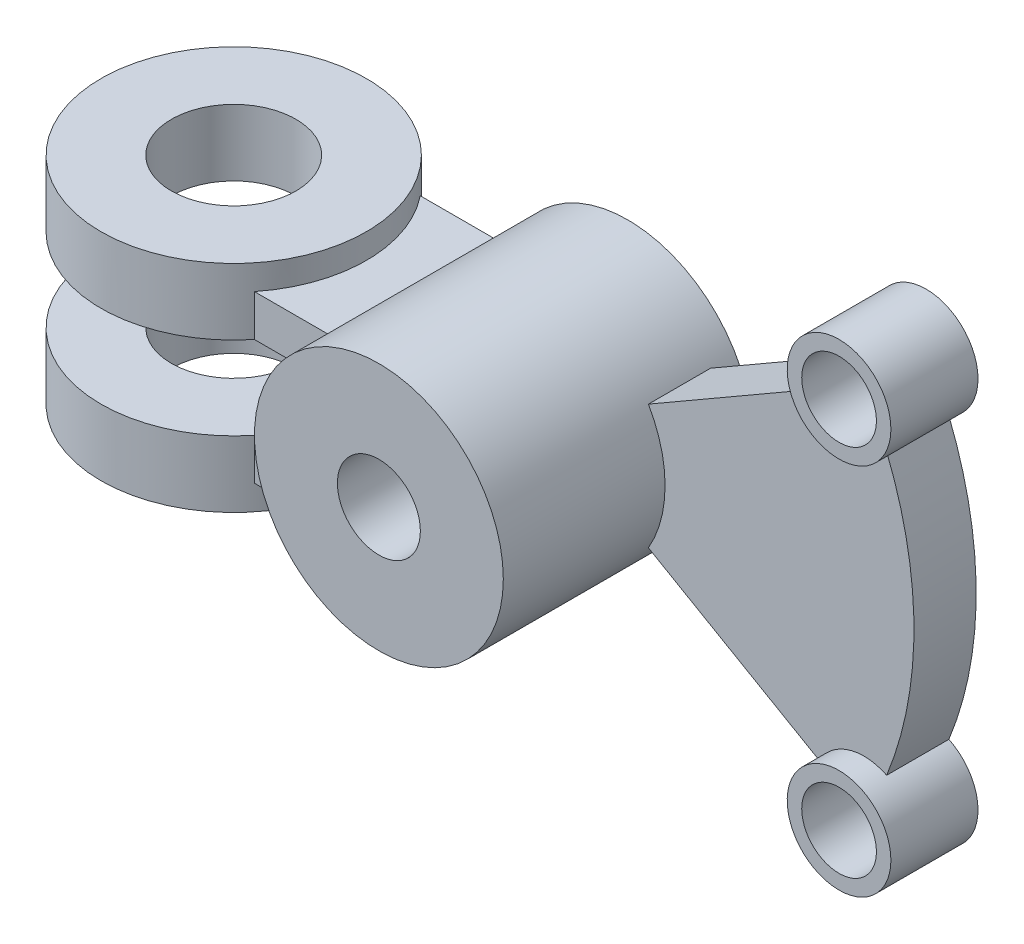
ISO-10303-21;
HEADER;
FILE_DESCRIPTION(('STEP AP214'),'2;1');
FILE_NAME('part.step','',(''),(''),'','','');
FILE_SCHEMA(('AUTOMOTIVE_DESIGN { 1 0 10303 214 1 1 1 1 }'));
ENDSEC;
DATA;
#1=APPLICATION_CONTEXT('core data for automotive mechanical design processes');
#2=APPLICATION_PROTOCOL_DEFINITION('international standard','automotive_design',2000,#1);
#3=PRODUCT_CONTEXT('',#1,'mechanical');
#4=PRODUCT('Part','Part','',(#3));
#5=PRODUCT_RELATED_PRODUCT_CATEGORY('part','',(#4));
#6=PRODUCT_DEFINITION_FORMATION('','',#4);
#7=PRODUCT_DEFINITION_CONTEXT('part definition',#1,'design');
#8=PRODUCT_DEFINITION('design','',#6,#7);
#9=PRODUCT_DEFINITION_SHAPE('','',#8);
#10=(LENGTH_UNIT() NAMED_UNIT(*) SI_UNIT(.MILLI.,.METRE.));
#11=(NAMED_UNIT(*) PLANE_ANGLE_UNIT() SI_UNIT($,.RADIAN.));
#12=(NAMED_UNIT(*) SI_UNIT($,.STERADIAN.) SOLID_ANGLE_UNIT());
#13=UNCERTAINTY_MEASURE_WITH_UNIT(LENGTH_MEASURE(1.E-05),#10,'distance_accuracy_value','');
#14=(GEOMETRIC_REPRESENTATION_CONTEXT(3) GLOBAL_UNCERTAINTY_ASSIGNED_CONTEXT((#13)) GLOBAL_UNIT_ASSIGNED_CONTEXT((#10,
#11,#12)) REPRESENTATION_CONTEXT('',''));
#15=CARTESIAN_POINT('',(0.,0.,0.));
#16=DIRECTION('',(0.,0.,1.));
#17=DIRECTION('',(1.,0.,0.));
#18=AXIS2_PLACEMENT_3D('',#15,#16,#17);
#19=CARTESIAN_POINT('',(0.,0.,21.));
#20=DIRECTION('',(0.,0.,-1.));
#21=DIRECTION('',(-1.,0.,0.));
#22=AXIS2_PLACEMENT_3D('',#19,#20,#21);
#23=CYLINDRICAL_SURFACE('',#22,90.);
#24=DIRECTION('',(0.,0.,-1.));
#25=VECTOR('',#24,1.);
#26=CARTESIAN_POINT('',(83.4254395553197,-33.7667889353089,16.5));
#27=LINE('',#26,#25);
#28=CARTESIAN_POINT('',(83.4254395553198,-33.7667889353088,6.));
#29=VERTEX_POINT('',#28);
#30=CARTESIAN_POINT('',(83.4254395553198,-33.7667889353088,21.));
#31=VERTEX_POINT('',#30);
#32=EDGE_CURVE('E374',#29,#31,#27,.F.);
#33=ORIENTED_EDGE('',*,*,#32,.F.);
#34=CARTESIAN_POINT('',(0.,0.,6.));
#35=DIRECTION('',(0.,0.,1.));
#36=DIRECTION('',(1.,0.,0.));
#37=AXIS2_PLACEMENT_3D('',#34,#35,#36);
#38=CIRCLE('',#37,90.);
#39=CARTESIAN_POINT('',(83.4254395553198,33.7667889353088,6.));
#40=VERTEX_POINT('',#39);
#41=EDGE_CURVE('E213',#29,#40,#38,.T.);
#42=ORIENTED_EDGE('',*,*,#41,.T.);
#43=DIRECTION('',(0.,0.,-1.));
#44=VECTOR('',#43,1.);
#45=CARTESIAN_POINT('',(83.4254395553198,33.7667889353089,16.5));
#46=LINE('',#45,#44);
#47=CARTESIAN_POINT('',(83.4254395553198,33.7667889353088,21.));
#48=VERTEX_POINT('',#47);
#49=EDGE_CURVE('E200',#48,#40,#46,.T.);
#50=ORIENTED_EDGE('',*,*,#49,.F.);
#51=CARTESIAN_POINT('',(0.,0.,21.));
#52=DIRECTION('',(0.,0.,1.));
#53=DIRECTION('',(1.,0.,0.));
#54=AXIS2_PLACEMENT_3D('',#51,#52,#53);
#55=CIRCLE('',#54,90.);
#56=EDGE_CURVE('E210',#31,#48,#55,.T.);
#57=ORIENTED_EDGE('',*,*,#56,.F.);
#58=EDGE_LOOP('',(#33,#42,#50,#57));
#59=FACE_BOUND('',#58,.T.);
#60=ADVANCED_FACE('F39',(#59),#23,.T.);
#61=CARTESIAN_POINT('',(0.,0.,21.));
#62=DIRECTION('',(0.500000000000001,0.866025403784438,0.));
#63=DIRECTION('',(-0.866025403784438,0.500000000000001,0.));
#64=AXIS2_PLACEMENT_3D('',#61,#62,#63);
#65=PLANE('',#64);
#66=DIRECTION('',(0.,0.,-1.));
#67=VECTOR('',#66,1.);
#68=CARTESIAN_POINT('',(67.116968793294,-38.7500000000001,27.));
#69=LINE('',#68,#67);
#70=CARTESIAN_POINT('',(67.116968793294,-38.7500000000001,21.));
#71=VERTEX_POINT('',#70);
#72=CARTESIAN_POINT('',(67.116968793294,-38.7500000000001,6.));
#73=VERTEX_POINT('',#72);
#74=EDGE_CURVE('E54',#71,#73,#69,.T.);
#75=ORIENTED_EDGE('',*,*,#74,.F.);
#76=DIRECTION('',(0.866025403784438,-0.500000000000001,0.));
#77=VECTOR('',#76,1.);
#78=CARTESIAN_POINT('',(0.,0.,21.));
#79=LINE('',#78,#77);
#80=CARTESIAN_POINT('',(25.9807621135331,-15.,21.));
#81=VERTEX_POINT('',#80);
#82=EDGE_CURVE('E201',#81,#71,#79,.T.);
#83=ORIENTED_EDGE('',*,*,#82,.F.);
#84=DIRECTION('',(0.,0.,-1.));
#85=VECTOR('',#84,1.);
#86=CARTESIAN_POINT('',(25.9807621135331,-15.,60.));
#87=LINE('',#86,#85);
#88=CARTESIAN_POINT('',(25.9807621135331,-15.,6.));
#89=VERTEX_POINT('',#88);
#90=EDGE_CURVE('E226',#81,#89,#87,.T.);
#91=ORIENTED_EDGE('',*,*,#90,.T.);
#92=DIRECTION('',(0.866025403784438,-0.500000000000001,0.));
#93=VECTOR('',#92,1.);
#94=CARTESIAN_POINT('',(0.,0.,6.));
#95=LINE('',#94,#93);
#96=EDGE_CURVE('E204',#89,#73,#95,.T.);
#97=ORIENTED_EDGE('',*,*,#96,.T.);
#98=EDGE_LOOP('',(#75,#83,#91,#97));
#99=FACE_BOUND('',#98,.T.);
#100=ADVANCED_FACE('F321',(#99),#65,.F.);
#101=CARTESIAN_POINT('',(-22.0435348575211,20.,50.));
#102=DIRECTION('',(0.,0.,-1.));
#103=DIRECTION('',(-1.,0.,0.));
#104=AXIS2_PLACEMENT_3D('',#101,#102,#103);
#105=PLANE('',#104);
#106=DIRECTION('',(0.,-1.,0.));
#107=VECTOR('',#106,1.);
#108=CARTESIAN_POINT('',(-40.0200080064064,26.,50.));
#109=LINE('',#108,#107);
#110=CARTESIAN_POINT('',(-40.0200080064064,10.,50.));
#111=VERTEX_POINT('',#110);
#112=CARTESIAN_POINT('',(-40.0200080064064,20.,50.));
#113=VERTEX_POINT('',#112);
#114=EDGE_CURVE('E167',#111,#113,#109,.F.);
#115=ORIENTED_EDGE('',*,*,#114,.F.);
#116=DIRECTION('',(1.,0.,0.));
#117=VECTOR('',#116,1.);
#118=CARTESIAN_POINT('',(-22.0435348575211,10.,50.));
#119=LINE('',#118,#117);
#120=CARTESIAN_POINT('',(-28.2842712474619,10.,50.));
#121=VERTEX_POINT('',#120);
#122=EDGE_CURVE('E181',#111,#121,#119,.T.);
#123=ORIENTED_EDGE('',*,*,#122,.T.);
#124=CARTESIAN_POINT('',(0.,0.,50.));
#125=DIRECTION('',(0.,0.,-1.));
#126=DIRECTION('',(-1.,0.,0.));
#127=AXIS2_PLACEMENT_3D('',#124,#125,#126);
#128=CIRCLE('',#127,30.);
#129=CARTESIAN_POINT('',(-22.3606797749979,20.,50.));
#130=VERTEX_POINT('',#129);
#131=EDGE_CURVE('E239',#121,#130,#128,.T.);
#132=ORIENTED_EDGE('',*,*,#131,.T.);
#133=DIRECTION('',(1.,0.,0.));
#134=VECTOR('',#133,1.);
#135=CARTESIAN_POINT('',(-80.,20.,50.));
#136=LINE('',#135,#134);
#137=EDGE_CURVE('E172',#113,#130,#136,.T.);
#138=ORIENTED_EDGE('',*,*,#137,.F.);
#139=EDGE_LOOP('',(#115,#123,#132,#138));
#140=FACE_BOUND('',#139,.T.);
#141=ADVANCED_FACE('F279',(#140),#105,.F.);
#142=CARTESIAN_POINT('',(-80.,20.,10.));
#143=DIRECTION('',(0.,0.,1.));
#144=DIRECTION('',(1.,0.,0.));
#145=AXIS2_PLACEMENT_3D('',#142,#143,#144);
#146=PLANE('',#145);
#147=DIRECTION('',(0.,-1.,0.));
#148=VECTOR('',#147,1.);
#149=CARTESIAN_POINT('',(-40.0200080064064,26.,9.99999999999999));
#150=LINE('',#149,#148);
#151=CARTESIAN_POINT('',(-40.0200080064064,20.,9.99999999999999));
#152=VERTEX_POINT('',#151);
#153=CARTESIAN_POINT('',(-40.0200080064064,10.,9.99999999999999));
#154=VERTEX_POINT('',#153);
#155=EDGE_CURVE('E48',#152,#154,#150,.T.);
#156=ORIENTED_EDGE('',*,*,#155,.F.);
#157=DIRECTION('',(-1.,0.,0.));
#158=VECTOR('',#157,1.);
#159=CARTESIAN_POINT('',(-29.7437728993575,20.,10.));
#160=LINE('',#159,#158);
#161=CARTESIAN_POINT('',(-22.3606797749979,20.,9.99999999999999));
#162=VERTEX_POINT('',#161);
#163=EDGE_CURVE('E176',#162,#152,#160,.T.);
#164=ORIENTED_EDGE('',*,*,#163,.F.);
#165=CARTESIAN_POINT('',(0.,0.,9.99999999999999));
#166=DIRECTION('',(0.,0.,1.));
#167=DIRECTION('',(1.,0.,0.));
#168=AXIS2_PLACEMENT_3D('',#165,#166,#167);
#169=CIRCLE('',#168,30.);
#170=CARTESIAN_POINT('',(-28.2842712474619,10.,9.99999999999999));
#171=VERTEX_POINT('',#170);
#172=EDGE_CURVE('E240',#162,#171,#169,.T.);
#173=ORIENTED_EDGE('',*,*,#172,.T.);
#174=DIRECTION('',(-1.,0.,0.));
#175=VECTOR('',#174,1.);
#176=CARTESIAN_POINT('',(-80.,10.,10.));
#177=LINE('',#176,#175);
#178=EDGE_CURVE('E180',#171,#154,#177,.T.);
#179=ORIENTED_EDGE('',*,*,#178,.T.);
#180=EDGE_LOOP('',(#156,#164,#173,#179));
#181=FACE_BOUND('',#180,.T.);
#182=ADVANCED_FACE('F272',(#181),#146,.F.);
#183=CARTESIAN_POINT('',(0.,0.,21.));
#184=DIRECTION('',(0.500000000000001,-0.866025403784438,0.));
#185=DIRECTION('',(0.866025403784438,0.500000000000001,0.));
#186=AXIS2_PLACEMENT_3D('',#183,#184,#185);
#187=PLANE('',#186);
#188=DIRECTION('',(0.,0.,-1.));
#189=VECTOR('',#188,1.);
#190=CARTESIAN_POINT('',(67.116968793294,38.7500000000001,27.));
#191=LINE('',#190,#189);
#192=CARTESIAN_POINT('',(67.116968793294,38.7500000000001,6.));
#193=VERTEX_POINT('',#192);
#194=CARTESIAN_POINT('',(67.116968793294,38.7500000000001,21.));
#195=VERTEX_POINT('',#194);
#196=EDGE_CURVE('E202',#193,#195,#191,.F.);
#197=ORIENTED_EDGE('',*,*,#196,.F.);
#198=DIRECTION('',(-0.866025403784438,-0.500000000000001,0.));
#199=VECTOR('',#198,1.);
#200=CARTESIAN_POINT('',(0.,0.,6.));
#201=LINE('',#200,#199);
#202=CARTESIAN_POINT('',(25.9807621135331,15.,6.));
#203=VERTEX_POINT('',#202);
#204=EDGE_CURVE('E206',#193,#203,#201,.T.);
#205=ORIENTED_EDGE('',*,*,#204,.T.);
#206=DIRECTION('',(0.,0.,-1.));
#207=VECTOR('',#206,1.);
#208=CARTESIAN_POINT('',(25.9807621135331,15.,60.));
#209=LINE('',#208,#207);
#210=CARTESIAN_POINT('',(25.9807621135331,15.,21.));
#211=VERTEX_POINT('',#210);
#212=EDGE_CURVE('E221',#203,#211,#209,.F.);
#213=ORIENTED_EDGE('',*,*,#212,.T.);
#214=DIRECTION('',(-0.866025403784438,-0.500000000000001,0.));
#215=VECTOR('',#214,1.);
#216=CARTESIAN_POINT('',(0.,0.,21.));
#217=LINE('',#216,#215);
#218=EDGE_CURVE('E208',#195,#211,#217,.T.);
#219=ORIENTED_EDGE('',*,*,#218,.F.);
#220=EDGE_LOOP('',(#197,#205,#213,#219));
#221=FACE_BOUND('',#220,.T.);
#222=ADVANCED_FACE('F327',(#221),#187,.F.);
#223=CARTESIAN_POINT('',(0.,0.,60.));
#224=DIRECTION('',(0.,0.,-1.));
#225=DIRECTION('',(-1.,0.,0.));
#226=AXIS2_PLACEMENT_3D('',#223,#224,#225);
#227=CYLINDRICAL_SURFACE('',#226,30.);
#228=CARTESIAN_POINT('',(0.,0.,50.));
#229=DIRECTION('',(0.,0.,1.));
#230=DIRECTION('',(1.,0.,0.));
#231=AXIS2_PLACEMENT_3D('',#228,#229,#230);
#232=CIRCLE('',#231,30.);
#233=CARTESIAN_POINT('',(-28.2842712474619,-10.,50.));
#234=VERTEX_POINT('',#233);
#235=CARTESIAN_POINT('',(-22.3606797749979,-20.,50.));
#236=VERTEX_POINT('',#235);
#237=EDGE_CURVE('E165',#234,#236,#232,.T.);
#238=ORIENTED_EDGE('',*,*,#237,.T.);
#239=DIRECTION('',(0.,0.,-1.));
#240=VECTOR('',#239,1.);
#241=CARTESIAN_POINT('',(-22.3606797749979,-20.,60.));
#242=LINE('',#241,#240);
#243=CARTESIAN_POINT('',(-22.3606797749979,-20.,9.99999999999999));
#244=VERTEX_POINT('',#243);
#245=EDGE_CURVE('E252',#236,#244,#242,.T.);
#246=ORIENTED_EDGE('',*,*,#245,.T.);
#247=CARTESIAN_POINT('',(0.,0.,9.99999999999999));
#248=DIRECTION('',(0.,0.,-1.));
#249=DIRECTION('',(-1.,0.,0.));
#250=AXIS2_PLACEMENT_3D('',#247,#248,#249);
#251=CIRCLE('',#250,30.);
#252=CARTESIAN_POINT('',(-28.2842712474619,-10.,10.));
#253=VERTEX_POINT('',#252);
#254=EDGE_CURVE('E248',#244,#253,#251,.T.);
#255=ORIENTED_EDGE('',*,*,#254,.T.);
#256=DIRECTION('',(0.,0.,-1.));
#257=VECTOR('',#256,1.);
#258=CARTESIAN_POINT('',(-28.2842712474619,-10.,60.));
#259=LINE('',#258,#257);
#260=EDGE_CURVE('E246',#234,#253,#259,.T.);
#261=ORIENTED_EDGE('',*,*,#260,.F.);
#262=EDGE_LOOP('',(#238,#246,#255,#261));
#263=FACE_BOUND('',#262,.T.);
#264=ORIENTED_EDGE('',*,*,#172,.F.);
#265=DIRECTION('',(0.,0.,-1.));
#266=VECTOR('',#265,1.);
#267=CARTESIAN_POINT('',(-22.3606797749979,20.,60.));
#268=LINE('',#267,#266);
#269=EDGE_CURVE('E243',#162,#130,#268,.F.);
#270=ORIENTED_EDGE('',*,*,#269,.T.);
#271=ORIENTED_EDGE('',*,*,#131,.F.);
#272=DIRECTION('',(0.,0.,-1.));
#273=VECTOR('',#272,1.);
#274=CARTESIAN_POINT('',(-28.2842712474619,10.,60.));
#275=LINE('',#274,#273);
#276=EDGE_CURVE('E234',#171,#121,#275,.F.);
#277=ORIENTED_EDGE('',*,*,#276,.F.);
#278=EDGE_LOOP('',(#264,#270,#271,#277));
#279=FACE_BOUND('',#278,.T.);
#280=ORIENTED_EDGE('',*,*,#90,.F.);
#281=CARTESIAN_POINT('',(0.,0.,21.));
#282=DIRECTION('',(0.,0.,1.));
#283=DIRECTION('',(1.,0.,0.));
#284=AXIS2_PLACEMENT_3D('',#281,#282,#283);
#285=CIRCLE('',#284,30.);
#286=EDGE_CURVE('E233',#81,#211,#285,.T.);
#287=ORIENTED_EDGE('',*,*,#286,.T.);
#288=ORIENTED_EDGE('',*,*,#212,.F.);
#289=CARTESIAN_POINT('',(0.,0.,6.));
#290=DIRECTION('',(0.,0.,1.));
#291=DIRECTION('',(1.,0.,0.));
#292=AXIS2_PLACEMENT_3D('',#289,#290,#291);
#293=CIRCLE('',#292,30.);
#294=EDGE_CURVE('E217',#89,#203,#293,.T.);
#295=ORIENTED_EDGE('',*,*,#294,.F.);
#296=EDGE_LOOP('',(#280,#287,#288,#295));
#297=FACE_BOUND('',#296,.T.);
#298=CARTESIAN_POINT('',(0.,0.,60.));
#299=DIRECTION('',(0.,0.,1.));
#300=DIRECTION('',(1.,0.,0.));
#301=AXIS2_PLACEMENT_3D('',#298,#299,#300);
#302=CIRCLE('',#301,30.);
#303=CARTESIAN_POINT('',(30.,0.,60.));
#304=VERTEX_POINT('',#303);
#305=EDGE_CURVE('E216',#304,#304,#302,.T.);
#306=ORIENTED_EDGE('',*,*,#305,.F.);
#307=EDGE_LOOP('',(#306));
#308=FACE_BOUND('',#307,.T.);
#309=CARTESIAN_POINT('',(0.,0.,0.));
#310=DIRECTION('',(0.,0.,1.));
#311=DIRECTION('',(1.,0.,0.));
#312=AXIS2_PLACEMENT_3D('',#309,#310,#311);
#313=CIRCLE('',#312,30.);
#314=CARTESIAN_POINT('',(30.,0.,0.));
#315=VERTEX_POINT('',#314);
#316=EDGE_CURVE('E215',#315,#315,#313,.T.);
#317=ORIENTED_EDGE('',*,*,#316,.T.);
#318=EDGE_LOOP('',(#317));
#319=FACE_BOUND('',#318,.T.);
#320=ADVANCED_FACE('F41',(#263,#279,#297,#308,#319),#227,.T.);
#321=CARTESIAN_POINT('',(0.,0.,60.));
#322=DIRECTION('',(0.,0.,1.));
#323=DIRECTION('',(1.,0.,0.));
#324=AXIS2_PLACEMENT_3D('',#321,#322,#323);
#325=PLANE('',#324);
#326=CARTESIAN_POINT('',(0.,0.,60.));
#327=DIRECTION('',(0.,0.,1.));
#328=DIRECTION('',(1.,0.,0.));
#329=AXIS2_PLACEMENT_3D('',#326,#327,#328);
#330=CIRCLE('',#329,10.);
#331=CARTESIAN_POINT('',(10.,0.,60.));
#332=VERTEX_POINT('',#331);
#333=EDGE_CURVE('E393',#332,#332,#330,.T.);
#334=ORIENTED_EDGE('',*,*,#333,.F.);
#335=EDGE_LOOP('',(#334));
#336=FACE_BOUND('',#335,.T.);
#337=ORIENTED_EDGE('',*,*,#305,.T.);
#338=EDGE_LOOP('',(#337));
#339=FACE_BOUND('',#338,.T.);
#340=ADVANCED_FACE('F333',(#336,#339),#325,.T.);
#341=CARTESIAN_POINT('',(0.,0.,0.));
#342=DIRECTION('',(0.,0.,1.));
#343=DIRECTION('',(1.,0.,0.));
#344=AXIS2_PLACEMENT_3D('',#341,#342,#343);
#345=PLANE('',#344);
#346=CARTESIAN_POINT('',(0.,0.,0.));
#347=DIRECTION('',(0.,0.,1.));
#348=DIRECTION('',(1.,0.,0.));
#349=AXIS2_PLACEMENT_3D('',#346,#347,#348);
#350=CIRCLE('',#349,10.);
#351=CARTESIAN_POINT('',(10.,0.,0.));
#352=VERTEX_POINT('',#351);
#353=EDGE_CURVE('E43',#352,#352,#350,.T.);
#354=ORIENTED_EDGE('',*,*,#353,.T.);
#355=EDGE_LOOP('',(#354));
#356=FACE_BOUND('',#355,.T.);
#357=ORIENTED_EDGE('',*,*,#316,.F.);
#358=EDGE_LOOP('',(#357));
#359=FACE_BOUND('',#358,.T.);
#360=ADVANCED_FACE('F331',(#356,#359),#345,.F.);
#361=CARTESIAN_POINT('',(0.,0.,21.));
#362=DIRECTION('',(0.,0.,1.));
#363=DIRECTION('',(1.,0.,0.));
#364=AXIS2_PLACEMENT_3D('',#361,#362,#363);
#365=PLANE('',#364);
#366=ORIENTED_EDGE('',*,*,#82,.T.);
#367=CARTESIAN_POINT('',(77.9422863405994,-45.0000000000001,21.));
#368=DIRECTION('',(0.,0.,1.));
#369=DIRECTION('',(1.,0.,0.));
#370=AXIS2_PLACEMENT_3D('',#367,#368,#369);
#371=CIRCLE('',#370,12.5);
#372=EDGE_CURVE('E65',#71,#31,#371,.F.);
#373=ORIENTED_EDGE('',*,*,#372,.T.);
#374=ORIENTED_EDGE('',*,*,#56,.T.);
#375=CARTESIAN_POINT('',(77.9422863405995,45.0000000000001,21.));
#376=DIRECTION('',(0.,0.,1.));
#377=DIRECTION('',(1.,0.,0.));
#378=AXIS2_PLACEMENT_3D('',#375,#376,#377);
#379=CIRCLE('',#378,12.5);
#380=EDGE_CURVE('E193',#48,#195,#379,.F.);
#381=ORIENTED_EDGE('',*,*,#380,.T.);
#382=ORIENTED_EDGE('',*,*,#218,.T.);
#383=ORIENTED_EDGE('',*,*,#286,.F.);
#384=EDGE_LOOP('',(#366,#373,#374,#381,#382,#383));
#385=FACE_BOUND('',#384,.T.);
#386=ADVANCED_FACE('F336',(#385),#365,.T.);
#387=CARTESIAN_POINT('',(0.,0.,6.));
#388=DIRECTION('',(0.,0.,1.));
#389=DIRECTION('',(1.,0.,0.));
#390=AXIS2_PLACEMENT_3D('',#387,#388,#389);
#391=PLANE('',#390);
#392=ORIENTED_EDGE('',*,*,#41,.F.);
#393=CARTESIAN_POINT('',(77.9422863405994,-45.0000000000001,6.));
#394=DIRECTION('',(0.,0.,1.));
#395=DIRECTION('',(1.,0.,0.));
#396=AXIS2_PLACEMENT_3D('',#393,#394,#395);
#397=CIRCLE('',#396,12.5);
#398=EDGE_CURVE('E377',#73,#29,#397,.T.);
#399=ORIENTED_EDGE('',*,*,#398,.F.);
#400=ORIENTED_EDGE('',*,*,#96,.F.);
#401=ORIENTED_EDGE('',*,*,#294,.T.);
#402=ORIENTED_EDGE('',*,*,#204,.F.);
#403=CARTESIAN_POINT('',(77.9422863405995,45.0000000000001,6.));
#404=DIRECTION('',(0.,0.,1.));
#405=DIRECTION('',(1.,0.,0.));
#406=AXIS2_PLACEMENT_3D('',#403,#404,#405);
#407=CIRCLE('',#406,12.5);
#408=EDGE_CURVE('E189',#40,#193,#407,.T.);
#409=ORIENTED_EDGE('',*,*,#408,.F.);
#410=EDGE_LOOP('',(#392,#399,#400,#401,#402,#409));
#411=FACE_BOUND('',#410,.T.);
#412=CARTESIAN_POINT('',(77.9422863405994,-45.0000000000001,6.));
#413=DIRECTION('',(0.,0.,1.));
#414=DIRECTION('',(1.,0.,0.));
#415=AXIS2_PLACEMENT_3D('',#412,#413,#414);
#416=CIRCLE('',#415,9.);
#417=CARTESIAN_POINT('',(68.9422863405994,-45.0000000000001,6.));
#418=VERTEX_POINT('',#417);
#419=EDGE_CURVE('E390',#418,#418,#416,.T.);
#420=ORIENTED_EDGE('',*,*,#419,.T.);
#421=EDGE_LOOP('',(#420));
#422=FACE_BOUND('',#421,.T.);
#423=CARTESIAN_POINT('',(77.9422863405995,45.0000000000001,6.));
#424=DIRECTION('',(0.,0.,1.));
#425=DIRECTION('',(1.,0.,0.));
#426=AXIS2_PLACEMENT_3D('',#423,#424,#425);
#427=CIRCLE('',#426,9.);
#428=CARTESIAN_POINT('',(68.9422863405995,45.0000000000001,6.));
#429=VERTEX_POINT('',#428);
#430=EDGE_CURVE('E179',#429,#429,#427,.T.);
#431=ORIENTED_EDGE('',*,*,#430,.T.);
#432=EDGE_LOOP('',(#431));
#433=FACE_BOUND('',#432,.T.);
#434=ADVANCED_FACE('F342',(#411,#422,#433),#391,.F.);
#435=CARTESIAN_POINT('',(77.9422863405995,45.0000000000001,27.));
#436=DIRECTION('',(0.,0.,-1.));
#437=DIRECTION('',(-1.,0.,0.));
#438=AXIS2_PLACEMENT_3D('',#435,#436,#437);
#439=CYLINDRICAL_SURFACE('',#438,12.5);
#440=CARTESIAN_POINT('',(77.9422863405995,45.0000000000001,27.));
#441=DIRECTION('',(0.,0.,1.));
#442=DIRECTION('',(1.,0.,0.));
#443=AXIS2_PLACEMENT_3D('',#440,#441,#442);
#444=CIRCLE('',#443,12.5);
#445=CARTESIAN_POINT('',(90.4422863405995,45.0000000000001,27.));
#446=VERTEX_POINT('',#445);
#447=EDGE_CURVE('E191',#446,#446,#444,.T.);
#448=ORIENTED_EDGE('',*,*,#447,.F.);
#449=EDGE_LOOP('',(#448));
#450=FACE_BOUND('',#449,.T.);
#451=ORIENTED_EDGE('',*,*,#408,.T.);
#452=ORIENTED_EDGE('',*,*,#196,.T.);
#453=ORIENTED_EDGE('',*,*,#380,.F.);
#454=ORIENTED_EDGE('',*,*,#49,.T.);
#455=EDGE_LOOP('',(#451,#452,#453,#454));
#456=FACE_BOUND('',#455,.T.);
#457=ADVANCED_FACE('F375',(#450,#456),#439,.T.);
#458=CARTESIAN_POINT('',(77.9422863405995,45.0000000000001,27.));
#459=DIRECTION('',(0.,0.,-1.));
#460=DIRECTION('',(-1.,0.,0.));
#461=AXIS2_PLACEMENT_3D('',#458,#459,#460);
#462=CYLINDRICAL_SURFACE('',#461,9.);
#463=CARTESIAN_POINT('',(77.9422863405995,45.0000000000001,27.));
#464=DIRECTION('',(0.,0.,1.));
#465=DIRECTION('',(1.,0.,0.));
#466=AXIS2_PLACEMENT_3D('',#463,#464,#465);
#467=CIRCLE('',#466,9.);
#468=CARTESIAN_POINT('',(68.9422863405995,45.0000000000001,27.));
#469=VERTEX_POINT('',#468);
#470=EDGE_CURVE('E184',#469,#469,#467,.T.);
#471=CARTESIAN_POINT('',(68.9422863405995,45.0000000000001,6.));
#472=CARTESIAN_POINT('',(68.9422863405995,45.0000000000001,6.21875));
#473=CARTESIAN_POINT('',(68.9422863405995,45.0000000000001,6.4375));
#474=CARTESIAN_POINT('',(68.9422863405995,45.0000000000001,6.875));
#475=CARTESIAN_POINT('',(68.9422863405995,45.0000000000001,7.09375));
#476=CARTESIAN_POINT('',(68.9422863405995,45.0000000000001,7.53125));
#477=CARTESIAN_POINT('',(68.9422863405995,45.0000000000001,7.75));
#478=CARTESIAN_POINT('',(68.9422863405995,45.0000000000001,8.1875));
#479=CARTESIAN_POINT('',(68.9422863405995,45.0000000000001,8.40625));
#480=CARTESIAN_POINT('',(68.9422863405995,45.0000000000001,8.84375));
#481=CARTESIAN_POINT('',(68.9422863405995,45.0000000000001,9.0625));
#482=CARTESIAN_POINT('',(68.9422863405995,45.0000000000001,9.5));
#483=CARTESIAN_POINT('',(68.9422863405995,45.0000000000001,9.71875));
#484=CARTESIAN_POINT('',(68.9422863405995,45.0000000000001,10.15625));
#485=CARTESIAN_POINT('',(68.9422863405995,45.0000000000001,10.375));
#486=CARTESIAN_POINT('',(68.9422863405995,45.0000000000001,10.8125));
#487=CARTESIAN_POINT('',(68.9422863405995,45.0000000000001,11.03125));
#488=CARTESIAN_POINT('',(68.9422863405995,45.0000000000001,11.46875));
#489=CARTESIAN_POINT('',(68.9422863405995,45.0000000000001,11.6875));
#490=CARTESIAN_POINT('',(68.9422863405995,45.0000000000001,12.125));
#491=CARTESIAN_POINT('',(68.9422863405995,45.0000000000001,12.34375));
#492=CARTESIAN_POINT('',(68.9422863405995,45.0000000000001,12.78125));
#493=CARTESIAN_POINT('',(68.9422863405995,45.0000000000001,13.));
#494=CARTESIAN_POINT('',(68.9422863405995,45.0000000000001,13.4375));
#495=CARTESIAN_POINT('',(68.9422863405995,45.0000000000001,13.65625));
#496=CARTESIAN_POINT('',(68.9422863405995,45.0000000000001,14.09375));
#497=CARTESIAN_POINT('',(68.9422863405995,45.0000000000001,14.3125));
#498=CARTESIAN_POINT('',(68.9422863405995,45.0000000000001,14.75));
#499=CARTESIAN_POINT('',(68.9422863405995,45.0000000000001,14.96875));
#500=CARTESIAN_POINT('',(68.9422863405995,45.0000000000001,15.40625));
#501=CARTESIAN_POINT('',(68.9422863405995,45.0000000000001,15.625));
#502=CARTESIAN_POINT('',(68.9422863405995,45.0000000000001,16.0625));
#503=CARTESIAN_POINT('',(68.9422863405995,45.0000000000001,16.28125));
#504=CARTESIAN_POINT('',(68.9422863405995,45.0000000000001,16.71875));
#505=CARTESIAN_POINT('',(68.9422863405995,45.0000000000001,16.9375));
#506=CARTESIAN_POINT('',(68.9422863405995,45.0000000000001,17.375));
#507=CARTESIAN_POINT('',(68.9422863405995,45.0000000000001,17.59375));
#508=CARTESIAN_POINT('',(68.9422863405995,45.0000000000001,18.03125));
#509=CARTESIAN_POINT('',(68.9422863405995,45.0000000000001,18.25));
#510=CARTESIAN_POINT('',(68.9422863405995,45.0000000000001,18.6875));
#511=CARTESIAN_POINT('',(68.9422863405995,45.0000000000001,18.90625));
#512=CARTESIAN_POINT('',(68.9422863405995,45.0000000000001,19.34375));
#513=CARTESIAN_POINT('',(68.9422863405995,45.0000000000001,19.5625));
#514=CARTESIAN_POINT('',(68.9422863405995,45.0000000000001,20.));
#515=CARTESIAN_POINT('',(68.9422863405995,45.0000000000001,20.21875));
#516=CARTESIAN_POINT('',(68.9422863405995,45.0000000000001,20.65625));
#517=CARTESIAN_POINT('',(68.9422863405995,45.0000000000001,20.875));
#518=CARTESIAN_POINT('',(68.9422863405995,45.0000000000001,21.3125));
#519=CARTESIAN_POINT('',(68.9422863405995,45.0000000000001,21.53125));
#520=CARTESIAN_POINT('',(68.9422863405995,45.0000000000001,21.96875));
#521=CARTESIAN_POINT('',(68.9422863405995,45.0000000000001,22.1875));
#522=CARTESIAN_POINT('',(68.9422863405995,45.0000000000001,22.625));
#523=CARTESIAN_POINT('',(68.9422863405995,45.0000000000001,22.84375));
#524=CARTESIAN_POINT('',(68.9422863405995,45.0000000000001,23.28125));
#525=CARTESIAN_POINT('',(68.9422863405995,45.0000000000001,23.5));
#526=CARTESIAN_POINT('',(68.9422863405995,45.0000000000001,23.9375));
#527=CARTESIAN_POINT('',(68.9422863405995,45.0000000000001,24.15625));
#528=CARTESIAN_POINT('',(68.9422863405995,45.0000000000001,24.59375));
#529=CARTESIAN_POINT('',(68.9422863405995,45.0000000000001,24.8125));
#530=CARTESIAN_POINT('',(68.9422863405995,45.0000000000001,25.25));
#531=CARTESIAN_POINT('',(68.9422863405995,45.0000000000001,25.46875));
#532=CARTESIAN_POINT('',(68.9422863405995,45.0000000000001,25.90625));
#533=CARTESIAN_POINT('',(68.9422863405995,45.0000000000001,26.125));
#534=CARTESIAN_POINT('',(68.9422863405995,45.0000000000001,26.5625));
#535=CARTESIAN_POINT('',(68.9422863405995,45.0000000000001,26.78125));
#536=CARTESIAN_POINT('',(68.9422863405995,45.0000000000001,27.));
#537=B_SPLINE_CURVE_WITH_KNOTS('',3,(#471,#472,#473,#474,#475,#476,#477,#478,#479,#480,#481,
#482,#483,#484,#485,#486,#487,#488,#489,#490,#491,#492,#493,#494,#495,#496,#497,#498,#499,#500,
#501,#502,#503,#504,#505,#506,#507,#508,#509,#510,#511,#512,#513,#514,#515,#516,#517,#518,#519,
#520,#521,#522,#523,#524,#525,#526,#527,#528,#529,#530,#531,#532,#533,#534,#535,#536),
.UNSPECIFIED.,.F.,.F.,(4,2,2,2,2,2,2,2,2,2,2,2,2,2,2,2,2,2,2,2,2,2,2,2,2,2,2,2,2,2,2,2,4),(0.,
0.656250000000001,1.3125,1.96875,2.625,3.28125,3.9375,4.59375,5.25,5.90625,6.5625,7.21875,7.875,
8.53125,9.1875,9.84375,10.5,11.15625,11.8125,12.46875,13.125,13.78125,14.4375,15.09375,15.75,
16.40625,17.0625,17.71875,18.375,19.03125,19.6875,20.34375,21.),.UNSPECIFIED.);
#538=EDGE_CURVE('BSEAM518',#429,#469,#537,.T.);
#539=ORIENTED_EDGE('',*,*,#430,.F.);
#540=ORIENTED_EDGE('',*,*,#470,.T.);
#541=ORIENTED_EDGE('',*,*,#538,.T.);
#542=ORIENTED_EDGE('',*,*,#538,.F.);
#543=EDGE_LOOP('',(#539,#541,#540,#542));
#544=FACE_BOUND('',#543,.T.);
#545=ADVANCED_FACE('F518',(#544),#462,.F.);
#546=CARTESIAN_POINT('',(77.9422863405995,45.0000000000001,27.));
#547=DIRECTION('',(0.,0.,1.));
#548=DIRECTION('',(1.,0.,0.));
#549=AXIS2_PLACEMENT_3D('',#546,#547,#548);
#550=PLANE('',#549);
#551=ORIENTED_EDGE('',*,*,#447,.T.);
#552=EDGE_LOOP('',(#551));
#553=FACE_BOUND('',#552,.T.);
#554=ORIENTED_EDGE('',*,*,#470,.F.);
#555=EDGE_LOOP('',(#554));
#556=FACE_BOUND('',#555,.T.);
#557=ADVANCED_FACE('F528',(#553,#556),#550,.T.);
#558=CARTESIAN_POINT('',(0.,20.,0.));
#559=DIRECTION('',(0.,1.,0.));
#560=DIRECTION('',(0.,0.,1.));
#561=AXIS2_PLACEMENT_3D('',#558,#559,#560);
#562=PLANE('',#561);
#563=ORIENTED_EDGE('',*,*,#163,.T.);
#564=CARTESIAN_POINT('',(-65.,20.,30.));
#565=DIRECTION('',(0.,1.,0.));
#566=DIRECTION('',(0.,0.,1.));
#567=AXIS2_PLACEMENT_3D('',#564,#565,#566);
#568=CIRCLE('',#567,32.);
#569=EDGE_CURVE('E259',#152,#113,#568,.F.);
#570=ORIENTED_EDGE('',*,*,#569,.T.);
#571=ORIENTED_EDGE('',*,*,#137,.T.);
#572=ORIENTED_EDGE('',*,*,#269,.F.);
#573=EDGE_LOOP('',(#563,#570,#571,#572));
#574=FACE_BOUND('',#573,.T.);
#575=ADVANCED_FACE('F280',(#574),#562,.T.);
#576=CARTESIAN_POINT('',(0.,10.,0.));
#577=DIRECTION('',(0.,1.,0.));
#578=DIRECTION('',(0.,0.,1.));
#579=AXIS2_PLACEMENT_3D('',#576,#577,#578);
#580=PLANE('',#579);
#581=ORIENTED_EDGE('',*,*,#122,.F.);
#582=CARTESIAN_POINT('',(-65.,10.,30.));
#583=DIRECTION('',(0.,1.,0.));
#584=DIRECTION('',(0.,0.,1.));
#585=AXIS2_PLACEMENT_3D('',#582,#583,#584);
#586=CIRCLE('',#585,32.);
#587=EDGE_CURVE('E260',#154,#111,#586,.T.);
#588=ORIENTED_EDGE('',*,*,#587,.F.);
#589=ORIENTED_EDGE('',*,*,#178,.F.);
#590=ORIENTED_EDGE('',*,*,#276,.T.);
#591=EDGE_LOOP('',(#581,#588,#589,#590));
#592=FACE_BOUND('',#591,.T.);
#593=CARTESIAN_POINT('',(-65.,10.,30.));
#594=DIRECTION('',(0.,1.,0.));
#595=DIRECTION('',(0.,0.,1.));
#596=AXIS2_PLACEMENT_3D('',#593,#594,#595);
#597=CIRCLE('',#596,15.);
#598=CARTESIAN_POINT('',(-65.,10.,45.));
#599=VERTEX_POINT('',#598);
#600=EDGE_CURVE('E292',#599,#599,#597,.T.);
#601=ORIENTED_EDGE('',*,*,#600,.T.);
#602=EDGE_LOOP('',(#601));
#603=FACE_BOUND('',#602,.T.);
#604=ADVANCED_FACE('F267',(#592,#603),#580,.F.);
#605=CARTESIAN_POINT('',(0.,-20.,0.));
#606=DIRECTION('',(0.,-1.,0.));
#607=DIRECTION('',(0.,0.,1.));
#608=AXIS2_PLACEMENT_3D('',#605,#606,#607);
#609=PLANE('',#608);
#610=CARTESIAN_POINT('',(-65.,-20.,30.));
#611=DIRECTION('',(0.,-1.,0.));
#612=DIRECTION('',(0.,0.,-1.));
#613=AXIS2_PLACEMENT_3D('',#610,#611,#612);
#614=CIRCLE('',#613,32.);
#615=CARTESIAN_POINT('',(-40.0200080064064,-20.,9.99999999999999));
#616=VERTEX_POINT('',#615);
#617=CARTESIAN_POINT('',(-40.0200080064064,-20.,50.));
#618=VERTEX_POINT('',#617);
#619=EDGE_CURVE('E143',#616,#618,#614,.T.);
#620=ORIENTED_EDGE('',*,*,#619,.F.);
#621=DIRECTION('',(-1.,0.,0.));
#622=VECTOR('',#621,1.);
#623=CARTESIAN_POINT('',(-80.,-20.,10.));
#624=LINE('',#623,#622);
#625=EDGE_CURVE('E164',#244,#616,#624,.T.);
#626=ORIENTED_EDGE('',*,*,#625,.F.);
#627=ORIENTED_EDGE('',*,*,#245,.F.);
#628=DIRECTION('',(1.,0.,0.));
#629=VECTOR('',#628,1.);
#630=CARTESIAN_POINT('',(-22.0435348575211,-20.,50.));
#631=LINE('',#630,#629);
#632=EDGE_CURVE('E166',#618,#236,#631,.T.);
#633=ORIENTED_EDGE('',*,*,#632,.F.);
#634=EDGE_LOOP('',(#620,#626,#627,#633));
#635=FACE_BOUND('',#634,.T.);
#636=ADVANCED_FACE('F288',(#635),#609,.T.);
#637=CARTESIAN_POINT('',(0.,-10.,0.));
#638=DIRECTION('',(0.,-1.,0.));
#639=DIRECTION('',(0.,0.,1.));
#640=AXIS2_PLACEMENT_3D('',#637,#638,#639);
#641=PLANE('',#640);
#642=DIRECTION('',(-1.,0.,0.));
#643=VECTOR('',#642,1.);
#644=CARTESIAN_POINT('',(-29.7437728993575,-10.,10.));
#645=LINE('',#644,#643);
#646=CARTESIAN_POINT('',(-40.0200080064064,-10.,9.99999999999999));
#647=VERTEX_POINT('',#646);
#648=EDGE_CURVE('E160',#253,#647,#645,.T.);
#649=ORIENTED_EDGE('',*,*,#648,.T.);
#650=CARTESIAN_POINT('',(-65.,-10.,30.));
#651=DIRECTION('',(0.,1.,0.));
#652=DIRECTION('',(0.,0.,1.));
#653=AXIS2_PLACEMENT_3D('',#650,#651,#652);
#654=CIRCLE('',#653,32.);
#655=CARTESIAN_POINT('',(-40.0200080064064,-10.,50.));
#656=VERTEX_POINT('',#655);
#657=EDGE_CURVE('E145',#647,#656,#654,.T.);
#658=ORIENTED_EDGE('',*,*,#657,.T.);
#659=DIRECTION('',(1.,0.,0.));
#660=VECTOR('',#659,1.);
#661=CARTESIAN_POINT('',(-80.,-10.,50.));
#662=LINE('',#661,#660);
#663=EDGE_CURVE('E153',#656,#234,#662,.T.);
#664=ORIENTED_EDGE('',*,*,#663,.T.);
#665=ORIENTED_EDGE('',*,*,#260,.T.);
#666=EDGE_LOOP('',(#649,#658,#664,#665));
#667=FACE_BOUND('',#666,.T.);
#668=CARTESIAN_POINT('',(-65.,-10.,30.));
#669=DIRECTION('',(0.,1.,0.));
#670=DIRECTION('',(0.,0.,1.));
#671=AXIS2_PLACEMENT_3D('',#668,#669,#670);
#672=CIRCLE('',#671,15.);
#673=CARTESIAN_POINT('',(-65.,-10.,45.));
#674=VERTEX_POINT('',#673);
#675=EDGE_CURVE('E399',#674,#674,#672,.T.);
#676=ORIENTED_EDGE('',*,*,#675,.F.);
#677=EDGE_LOOP('',(#676));
#678=FACE_BOUND('',#677,.T.);
#679=ADVANCED_FACE('F154',(#667,#678),#641,.F.);
#680=CARTESIAN_POINT('',(-29.7437728993575,-20.,10.));
#681=DIRECTION('',(0.,0.,-1.));
#682=DIRECTION('',(-1.,0.,0.));
#683=AXIS2_PLACEMENT_3D('',#680,#681,#682);
#684=PLANE('',#683);
#685=DIRECTION('',(0.,1.,0.));
#686=VECTOR('',#685,1.);
#687=CARTESIAN_POINT('',(-40.0200080064064,-26.,9.99999999999999));
#688=LINE('',#687,#686);
#689=EDGE_CURVE('E293',#647,#616,#688,.F.);
#690=ORIENTED_EDGE('',*,*,#689,.F.);
#691=ORIENTED_EDGE('',*,*,#648,.F.);
#692=ORIENTED_EDGE('',*,*,#254,.F.);
#693=ORIENTED_EDGE('',*,*,#625,.T.);
#694=EDGE_LOOP('',(#690,#691,#692,#693));
#695=FACE_BOUND('',#694,.T.);
#696=ADVANCED_FACE('F286',(#695),#684,.T.);
#697=CARTESIAN_POINT('',(-80.,-20.,50.));
#698=DIRECTION('',(0.,0.,1.));
#699=DIRECTION('',(1.,0.,0.));
#700=AXIS2_PLACEMENT_3D('',#697,#698,#699);
#701=PLANE('',#700);
#702=DIRECTION('',(0.,1.,0.));
#703=VECTOR('',#702,1.);
#704=CARTESIAN_POINT('',(-40.0200080064064,-26.,50.));
#705=LINE('',#704,#703);
#706=EDGE_CURVE('E11',#618,#656,#705,.T.);
#707=ORIENTED_EDGE('',*,*,#706,.F.);
#708=ORIENTED_EDGE('',*,*,#632,.T.);
#709=ORIENTED_EDGE('',*,*,#237,.F.);
#710=ORIENTED_EDGE('',*,*,#663,.F.);
#711=EDGE_LOOP('',(#707,#708,#709,#710));
#712=FACE_BOUND('',#711,.T.);
#713=ADVANCED_FACE('F162',(#712),#701,.T.);
#714=CARTESIAN_POINT('',(-65.,26.,30.));
#715=DIRECTION('',(0.,-1.,0.));
#716=DIRECTION('',(0.,0.,-1.));
#717=AXIS2_PLACEMENT_3D('',#714,#715,#716);
#718=CYLINDRICAL_SURFACE('',#717,32.);
#719=CARTESIAN_POINT('',(-65.,26.,30.));
#720=DIRECTION('',(0.,1.,0.));
#721=DIRECTION('',(0.,0.,1.));
#722=AXIS2_PLACEMENT_3D('',#719,#720,#721);
#723=CIRCLE('',#722,32.);
#724=CARTESIAN_POINT('',(-65.,26.,62.));
#725=VERTEX_POINT('',#724);
#726=EDGE_CURVE('E268',#725,#725,#723,.T.);
#727=ORIENTED_EDGE('',*,*,#726,.F.);
#728=EDGE_LOOP('',(#727));
#729=FACE_BOUND('',#728,.T.);
#730=ORIENTED_EDGE('',*,*,#587,.T.);
#731=ORIENTED_EDGE('',*,*,#114,.T.);
#732=ORIENTED_EDGE('',*,*,#569,.F.);
#733=ORIENTED_EDGE('',*,*,#155,.T.);
#734=EDGE_LOOP('',(#730,#731,#732,#733));
#735=FACE_BOUND('',#734,.T.);
#736=ADVANCED_FACE('F256',(#729,#735),#718,.T.);
#737=CARTESIAN_POINT('',(-65.,26.,30.));
#738=DIRECTION('',(0.,-1.,0.));
#739=DIRECTION('',(0.,0.,-1.));
#740=AXIS2_PLACEMENT_3D('',#737,#738,#739);
#741=CYLINDRICAL_SURFACE('',#740,15.);
#742=CARTESIAN_POINT('',(-65.,26.,30.));
#743=DIRECTION('',(0.,1.,0.));
#744=DIRECTION('',(0.,0.,1.));
#745=AXIS2_PLACEMENT_3D('',#742,#743,#744);
#746=CIRCLE('',#745,15.);
#747=CARTESIAN_POINT('',(-65.,26.,45.));
#748=VERTEX_POINT('',#747);
#749=EDGE_CURVE('E269',#748,#748,#746,.T.);
#750=ORIENTED_EDGE('',*,*,#749,.T.);
#751=EDGE_LOOP('',(#750));
#752=FACE_BOUND('',#751,.T.);
#753=ORIENTED_EDGE('',*,*,#600,.F.);
#754=EDGE_LOOP('',(#753));
#755=FACE_BOUND('',#754,.T.);
#756=ADVANCED_FACE('F310',(#752,#755),#741,.F.);
#757=CARTESIAN_POINT('',(-65.,26.,30.));
#758=DIRECTION('',(0.,1.,0.));
#759=DIRECTION('',(0.,0.,1.));
#760=AXIS2_PLACEMENT_3D('',#757,#758,#759);
#761=PLANE('',#760);
#762=ORIENTED_EDGE('',*,*,#726,.T.);
#763=EDGE_LOOP('',(#762));
#764=FACE_BOUND('',#763,.T.);
#765=ORIENTED_EDGE('',*,*,#749,.F.);
#766=EDGE_LOOP('',(#765));
#767=FACE_BOUND('',#766,.T.);
#768=ADVANCED_FACE('F303',(#764,#767),#761,.T.);
#769=CARTESIAN_POINT('',(-65.,-26.,30.));
#770=DIRECTION('',(0.,1.,0.));
#771=DIRECTION('',(0.,0.,1.));
#772=AXIS2_PLACEMENT_3D('',#769,#770,#771);
#773=CYLINDRICAL_SURFACE('',#772,32.);
#774=CARTESIAN_POINT('',(-65.,-26.,30.));
#775=DIRECTION('',(0.,1.,0.));
#776=DIRECTION('',(0.,0.,1.));
#777=AXIS2_PLACEMENT_3D('',#774,#775,#776);
#778=CIRCLE('',#777,32.);
#779=CARTESIAN_POINT('',(-65.,-26.,62.));
#780=VERTEX_POINT('',#779);
#781=EDGE_CURVE('E158',#780,#780,#778,.T.);
#782=ORIENTED_EDGE('',*,*,#781,.T.);
#783=EDGE_LOOP('',(#782));
#784=FACE_BOUND('',#783,.T.);
#785=ORIENTED_EDGE('',*,*,#657,.F.);
#786=ORIENTED_EDGE('',*,*,#689,.T.);
#787=ORIENTED_EDGE('',*,*,#619,.T.);
#788=ORIENTED_EDGE('',*,*,#706,.T.);
#789=EDGE_LOOP('',(#785,#786,#787,#788));
#790=FACE_BOUND('',#789,.T.);
#791=ADVANCED_FACE('F142',(#784,#790),#773,.T.);
#792=CARTESIAN_POINT('',(-65.,-26.,30.));
#793=DIRECTION('',(0.,-1.,0.));
#794=DIRECTION('',(0.,0.,1.));
#795=AXIS2_PLACEMENT_3D('',#792,#793,#794);
#796=PLANE('',#795);
#797=CARTESIAN_POINT('',(-65.,-26.,30.));
#798=DIRECTION('',(0.,1.,0.));
#799=DIRECTION('',(0.,0.,1.));
#800=AXIS2_PLACEMENT_3D('',#797,#798,#799);
#801=CIRCLE('',#800,15.);
#802=CARTESIAN_POINT('',(-65.,-26.,45.));
#803=VERTEX_POINT('',#802);
#804=EDGE_CURVE('E159',#803,#803,#801,.T.);
#805=ORIENTED_EDGE('',*,*,#804,.T.);
#806=EDGE_LOOP('',(#805));
#807=FACE_BOUND('',#806,.T.);
#808=ORIENTED_EDGE('',*,*,#781,.F.);
#809=EDGE_LOOP('',(#808));
#810=FACE_BOUND('',#809,.T.);
#811=ADVANCED_FACE('F406',(#807,#810),#796,.T.);
#812=CARTESIAN_POINT('',(-65.,-26.,30.));
#813=DIRECTION('',(0.,1.,0.));
#814=DIRECTION('',(0.,0.,1.));
#815=AXIS2_PLACEMENT_3D('',#812,#813,#814);
#816=CYLINDRICAL_SURFACE('',#815,15.);
#817=ORIENTED_EDGE('',*,*,#675,.T.);
#818=EDGE_LOOP('',(#817));
#819=FACE_BOUND('',#818,.T.);
#820=ORIENTED_EDGE('',*,*,#804,.F.);
#821=EDGE_LOOP('',(#820));
#822=FACE_BOUND('',#821,.T.);
#823=ADVANCED_FACE('F407',(#819,#822),#816,.F.);
#824=CARTESIAN_POINT('',(0.,0.,-2.00000000000001));
#825=DIRECTION('',(0.,0.,1.));
#826=DIRECTION('',(1.,0.,0.));
#827=AXIS2_PLACEMENT_3D('',#824,#825,#826);
#828=CYLINDRICAL_SURFACE('',#827,10.);
#829=ORIENTED_EDGE('',*,*,#333,.T.);
#830=EDGE_LOOP('',(#829));
#831=FACE_BOUND('',#830,.T.);
#832=ORIENTED_EDGE('',*,*,#353,.F.);
#833=EDGE_LOOP('',(#832));
#834=FACE_BOUND('',#833,.T.);
#835=ADVANCED_FACE('F417',(#831,#834),#828,.F.);
#836=CARTESIAN_POINT('',(77.9422863405994,-45.0000000000001,27.));
#837=DIRECTION('',(0.,0.,-1.));
#838=DIRECTION('',(-1.,0.,0.));
#839=AXIS2_PLACEMENT_3D('',#836,#837,#838);
#840=CYLINDRICAL_SURFACE('',#839,12.5);
#841=CARTESIAN_POINT('',(77.9422863405994,-45.0000000000001,27.));
#842=DIRECTION('',(0.,0.,1.));
#843=DIRECTION('',(1.,0.,0.));
#844=AXIS2_PLACEMENT_3D('',#841,#842,#843);
#845=CIRCLE('',#844,12.5);
#846=CARTESIAN_POINT('',(90.4422863405994,-45.0000000000001,27.));
#847=VERTEX_POINT('',#846);
#848=EDGE_CURVE('E382',#847,#847,#845,.T.);
#849=ORIENTED_EDGE('',*,*,#848,.F.);
#850=EDGE_LOOP('',(#849));
#851=FACE_BOUND('',#850,.T.);
#852=ORIENTED_EDGE('',*,*,#398,.T.);
#853=ORIENTED_EDGE('',*,*,#32,.T.);
#854=ORIENTED_EDGE('',*,*,#372,.F.);
#855=ORIENTED_EDGE('',*,*,#74,.T.);
#856=EDGE_LOOP('',(#852,#853,#854,#855));
#857=FACE_BOUND('',#856,.T.);
#858=ADVANCED_FACE('F379',(#851,#857),#840,.T.);
#859=CARTESIAN_POINT('',(77.9422863405994,-45.0000000000001,27.));
#860=DIRECTION('',(0.,0.,-1.));
#861=DIRECTION('',(-1.,0.,0.));
#862=AXIS2_PLACEMENT_3D('',#859,#860,#861);
#863=CYLINDRICAL_SURFACE('',#862,9.);
#864=CARTESIAN_POINT('',(77.9422863405994,-45.0000000000001,27.));
#865=DIRECTION('',(0.,0.,1.));
#866=DIRECTION('',(1.,0.,0.));
#867=AXIS2_PLACEMENT_3D('',#864,#865,#866);
#868=CIRCLE('',#867,9.);
#869=CARTESIAN_POINT('',(68.9422863405994,-45.0000000000001,27.));
#870=VERTEX_POINT('',#869);
#871=EDGE_CURVE('E385',#870,#870,#868,.T.);
#872=CARTESIAN_POINT('',(68.9422863405994,-45.0000000000001,6.));
#873=CARTESIAN_POINT('',(68.9422863405994,-45.0000000000001,6.21875));
#874=CARTESIAN_POINT('',(68.9422863405994,-45.0000000000001,6.4375));
#875=CARTESIAN_POINT('',(68.9422863405994,-45.0000000000001,6.875));
#876=CARTESIAN_POINT('',(68.9422863405994,-45.0000000000001,7.09375));
#877=CARTESIAN_POINT('',(68.9422863405994,-45.0000000000001,7.53125));
#878=CARTESIAN_POINT('',(68.9422863405994,-45.0000000000001,7.75));
#879=CARTESIAN_POINT('',(68.9422863405994,-45.0000000000001,8.1875));
#880=CARTESIAN_POINT('',(68.9422863405994,-45.0000000000001,8.40625));
#881=CARTESIAN_POINT('',(68.9422863405994,-45.0000000000001,8.84375));
#882=CARTESIAN_POINT('',(68.9422863405994,-45.0000000000001,9.0625));
#883=CARTESIAN_POINT('',(68.9422863405994,-45.0000000000001,9.5));
#884=CARTESIAN_POINT('',(68.9422863405994,-45.0000000000001,9.71875));
#885=CARTESIAN_POINT('',(68.9422863405994,-45.0000000000001,10.15625));
#886=CARTESIAN_POINT('',(68.9422863405994,-45.0000000000001,10.375));
#887=CARTESIAN_POINT('',(68.9422863405994,-45.0000000000001,10.8125));
#888=CARTESIAN_POINT('',(68.9422863405994,-45.0000000000001,11.03125));
#889=CARTESIAN_POINT('',(68.9422863405994,-45.0000000000001,11.46875));
#890=CARTESIAN_POINT('',(68.9422863405994,-45.0000000000001,11.6875));
#891=CARTESIAN_POINT('',(68.9422863405994,-45.0000000000001,12.125));
#892=CARTESIAN_POINT('',(68.9422863405994,-45.0000000000001,12.34375));
#893=CARTESIAN_POINT('',(68.9422863405994,-45.0000000000001,12.78125));
#894=CARTESIAN_POINT('',(68.9422863405994,-45.0000000000001,13.));
#895=CARTESIAN_POINT('',(68.9422863405994,-45.0000000000001,13.4375));
#896=CARTESIAN_POINT('',(68.9422863405994,-45.0000000000001,13.65625));
#897=CARTESIAN_POINT('',(68.9422863405994,-45.0000000000001,14.09375));
#898=CARTESIAN_POINT('',(68.9422863405994,-45.0000000000001,14.3125));
#899=CARTESIAN_POINT('',(68.9422863405994,-45.0000000000001,14.75));
#900=CARTESIAN_POINT('',(68.9422863405994,-45.0000000000001,14.96875));
#901=CARTESIAN_POINT('',(68.9422863405994,-45.0000000000001,15.40625));
#902=CARTESIAN_POINT('',(68.9422863405994,-45.0000000000001,15.625));
#903=CARTESIAN_POINT('',(68.9422863405994,-45.0000000000001,16.0625));
#904=CARTESIAN_POINT('',(68.9422863405994,-45.0000000000001,16.28125));
#905=CARTESIAN_POINT('',(68.9422863405994,-45.0000000000001,16.71875));
#906=CARTESIAN_POINT('',(68.9422863405994,-45.0000000000001,16.9375));
#907=CARTESIAN_POINT('',(68.9422863405994,-45.0000000000001,17.375));
#908=CARTESIAN_POINT('',(68.9422863405994,-45.0000000000001,17.59375));
#909=CARTESIAN_POINT('',(68.9422863405994,-45.0000000000001,18.03125));
#910=CARTESIAN_POINT('',(68.9422863405994,-45.0000000000001,18.25));
#911=CARTESIAN_POINT('',(68.9422863405994,-45.0000000000001,18.6875));
#912=CARTESIAN_POINT('',(68.9422863405994,-45.0000000000001,18.90625));
#913=CARTESIAN_POINT('',(68.9422863405994,-45.0000000000001,19.34375));
#914=CARTESIAN_POINT('',(68.9422863405994,-45.0000000000001,19.5625));
#915=CARTESIAN_POINT('',(68.9422863405994,-45.0000000000001,20.));
#916=CARTESIAN_POINT('',(68.9422863405994,-45.0000000000001,20.21875));
#917=CARTESIAN_POINT('',(68.9422863405994,-45.0000000000001,20.65625));
#918=CARTESIAN_POINT('',(68.9422863405994,-45.0000000000001,20.875));
#919=CARTESIAN_POINT('',(68.9422863405994,-45.0000000000001,21.3125));
#920=CARTESIAN_POINT('',(68.9422863405994,-45.0000000000001,21.53125));
#921=CARTESIAN_POINT('',(68.9422863405994,-45.0000000000001,21.96875));
#922=CARTESIAN_POINT('',(68.9422863405994,-45.0000000000001,22.1875));
#923=CARTESIAN_POINT('',(68.9422863405994,-45.0000000000001,22.625));
#924=CARTESIAN_POINT('',(68.9422863405994,-45.0000000000001,22.84375));
#925=CARTESIAN_POINT('',(68.9422863405994,-45.0000000000001,23.28125));
#926=CARTESIAN_POINT('',(68.9422863405994,-45.0000000000001,23.5));
#927=CARTESIAN_POINT('',(68.9422863405994,-45.0000000000001,23.9375));
#928=CARTESIAN_POINT('',(68.9422863405994,-45.0000000000001,24.15625));
#929=CARTESIAN_POINT('',(68.9422863405994,-45.0000000000001,24.59375));
#930=CARTESIAN_POINT('',(68.9422863405994,-45.0000000000001,24.8125));
#931=CARTESIAN_POINT('',(68.9422863405994,-45.0000000000001,25.25));
#932=CARTESIAN_POINT('',(68.9422863405994,-45.0000000000001,25.46875));
#933=CARTESIAN_POINT('',(68.9422863405994,-45.0000000000001,25.90625));
#934=CARTESIAN_POINT('',(68.9422863405994,-45.0000000000001,26.125));
#935=CARTESIAN_POINT('',(68.9422863405994,-45.0000000000001,26.5625));
#936=CARTESIAN_POINT('',(68.9422863405994,-45.0000000000001,26.78125));
#937=CARTESIAN_POINT('',(68.9422863405994,-45.0000000000001,27.));
#938=B_SPLINE_CURVE_WITH_KNOTS('',3,(#872,#873,#874,#875,#876,#877,#878,#879,#880,#881,#882,
#883,#884,#885,#886,#887,#888,#889,#890,#891,#892,#893,#894,#895,#896,#897,#898,#899,#900,#901,
#902,#903,#904,#905,#906,#907,#908,#909,#910,#911,#912,#913,#914,#915,#916,#917,#918,#919,#920,
#921,#922,#923,#924,#925,#926,#927,#928,#929,#930,#931,#932,#933,#934,#935,#936,#937),
.UNSPECIFIED.,.F.,.F.,(4,2,2,2,2,2,2,2,2,2,2,2,2,2,2,2,2,2,2,2,2,2,2,2,2,2,2,2,2,2,2,2,4),(0.,
0.656250000000001,1.3125,1.96875,2.625,3.28125,3.9375,4.59375,5.25,5.90625,6.5625,7.21875,7.875,
8.53125,9.1875,9.84375,10.5,11.15625,11.8125,12.46875,13.125,13.78125,14.4375,15.09375,15.75,
16.40625,17.0625,17.71875,18.375,19.03125,19.6875,20.34375,21.),.UNSPECIFIED.);
#939=EDGE_CURVE('BSEAM620',#418,#870,#938,.T.);
#940=ORIENTED_EDGE('',*,*,#419,.F.);
#941=ORIENTED_EDGE('',*,*,#871,.T.);
#942=ORIENTED_EDGE('',*,*,#939,.T.);
#943=ORIENTED_EDGE('',*,*,#939,.F.);
#944=EDGE_LOOP('',(#940,#942,#941,#943));
#945=FACE_BOUND('',#944,.T.);
#946=ADVANCED_FACE('F620',(#945),#863,.F.);
#947=CARTESIAN_POINT('',(77.9422863405994,-45.0000000000001,27.));
#948=DIRECTION('',(0.,0.,1.));
#949=DIRECTION('',(1.,0.,0.));
#950=AXIS2_PLACEMENT_3D('',#947,#948,#949);
#951=PLANE('',#950);
#952=ORIENTED_EDGE('',*,*,#848,.T.);
#953=EDGE_LOOP('',(#952));
#954=FACE_BOUND('',#953,.T.);
#955=ORIENTED_EDGE('',*,*,#871,.F.);
#956=EDGE_LOOP('',(#955));
#957=FACE_BOUND('',#956,.T.);
#958=ADVANCED_FACE('F627',(#954,#957),#951,.T.);
#959=CLOSED_SHELL('',(#60,#100,#141,#182,#222,#320,#340,#360,#386,#434,#457,#545,#557,#575,#604,
#636,#679,#696,#713,#736,#756,#768,#791,#811,#823,#835,#858,#946,#958));
#960=MANIFOLD_SOLID_BREP('B2',#959);
#961=ADVANCED_BREP_SHAPE_REPRESENTATION('',(#18,#960),#14);
#962=SHAPE_DEFINITION_REPRESENTATION(#9,#961);
ENDSEC;
END-ISO-10303-21;
